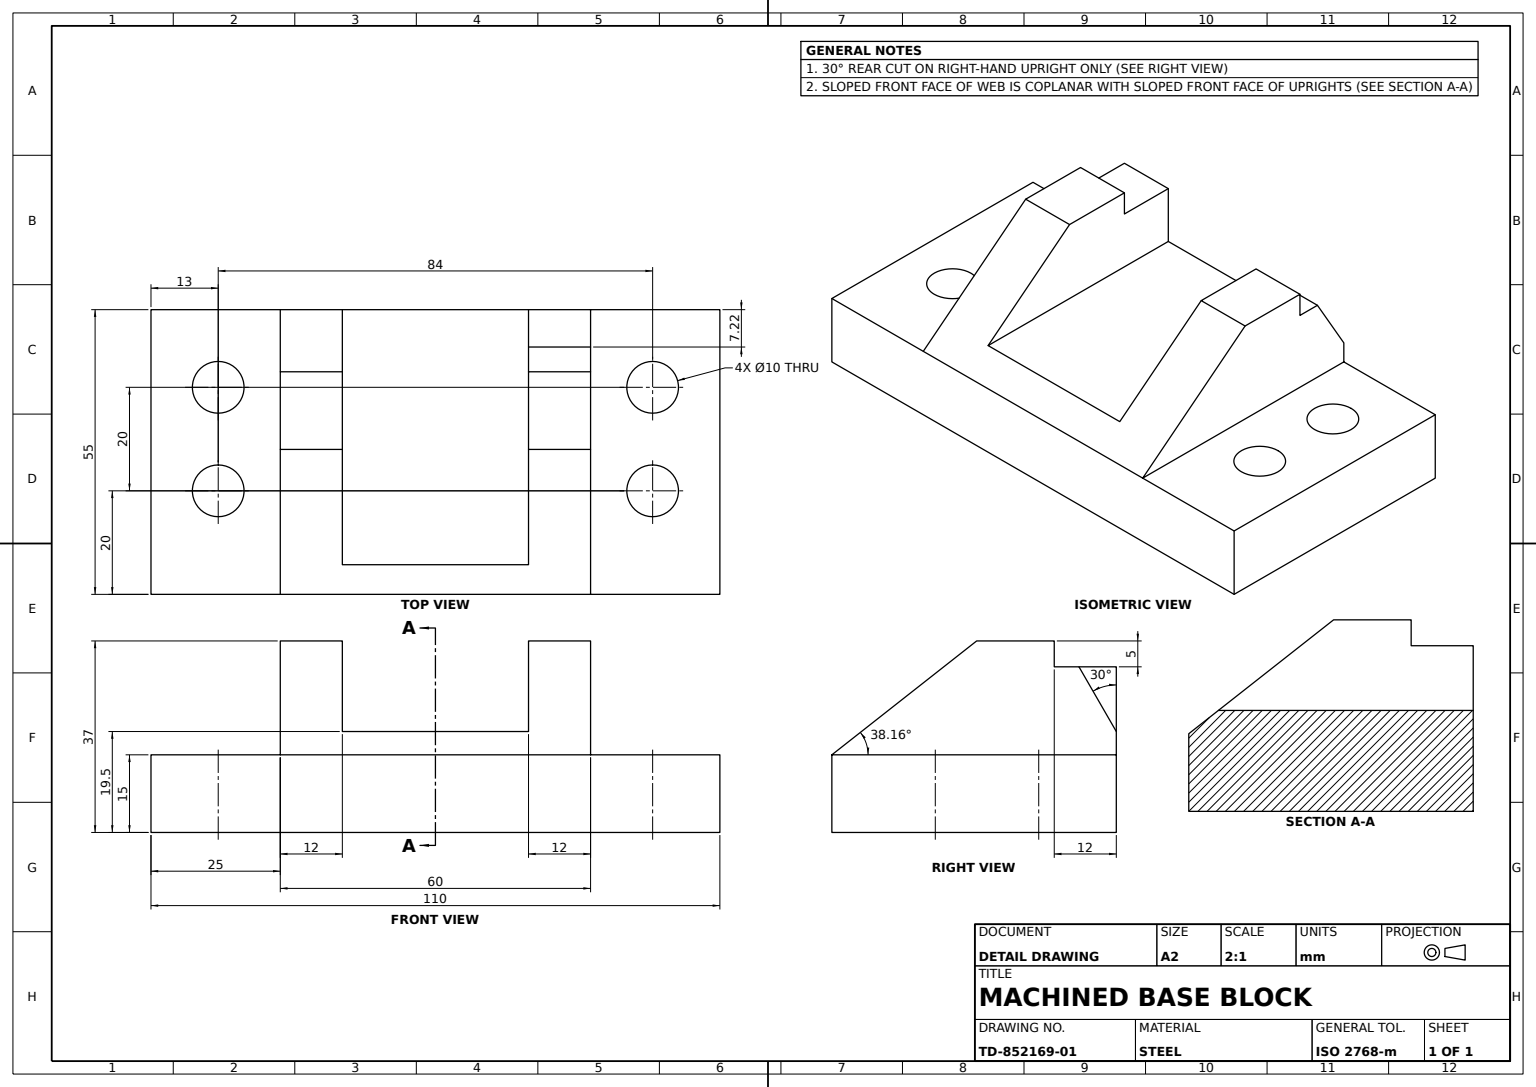
SolidWorks part; units mm, degrees
material "Plain Carbon Steel"
ref_plane "Front Plane" through (0, 0, 0) normal (0, 0, 1) x (1, 0, 0)
ref_plane "Top Plane" through (0, 0, 0) normal (0, 1, 0) x (1, 0, 0)
ref_plane "Right Plane" through (0, 0, 0) normal (1, 0, 0) x (0, 0, -1)
sketch "Base Plate Sketch" plane through (0, 0, 0) normal (0, 1, 0) x (1, 0, 0)
  line L0 (0, 55) -> (0, 0) construction
  line L1 (-55, 0) -> (55, 0)
  line L2 (-55, 0) -> (-55, 55)
  line L3 (-55, 55) -> (55, 55)
  line L4 (55, 0) -> (55, 55)
  line L5 (-42, 55) -> (-42, 0) construction
  circle A0 centre (-42, 40) radius 5
  circle A1 centre (-42, 20) radius 5
  circle A2 centre (42, 20) radius 5
  circle A3 centre (42, 40) radius 5
  point P4 (0, 0)
  dimension "D3" = 20
  dimension "D4" = 10
  dimension "D1" = 110
  dimension "D2" = 55
  dimension "D5" = 20
  dimension "D6" = 42
extrude "Base Plate" add sketch "Base Plate Sketch" along normal blind 15
sketch "V-Block Uprights Sketch" plane through (0, 0, -55) normal (0, 0, -1) x (-1, 0, 0)
  line L0 (0, 15) -> (0, 63.744) construction
  line L1 (-55, 15) -> (55, 15) construction
  line L2 (-30, 37) -> (30, 37) construction
  line L3 (-30, 15) -> (-18, 15)
  line L4 (-30, 15) -> (-30, 37)
  line L5 (-30, 37) -> (-18, 37)
  line L6 (-18, 19.5) -> (-18, 37)
  line L7 (18, 15) -> (30, 15)
  line L8 (18, 19.5) -> (18, 37)
  line L9 (18, 37) -> (30, 37)
  line L10 (30, 15) -> (30, 37)
  line L11 (18, 19.5) -> (-18, 19.5)
  line L12 (18, 15) -> (-18, 15)
  line L14 (-55, 0) -> (55, 0) construction
  circle A0 centre (0, 37) radius 17.5 construction
  point P18 (0, 19.5)
  point P20 (0, 15)
  dimension "D5" = 35
  dimension "D1" = 22
  dimension "D2" = 12
  dimension "D3" = 12
  dimension "D4" = 60
  dimension "D6" = 19.5
extrude "V-Block Uprights" add sketch "V-Block Uprights Sketch" against normal up to surface (55 mm away) up to face at (0, 7.5, 0)
sketch "Upright Notch Sketch" plane through (-30, 0, 0) normal (-1, 0, 0) x (0, 0, 1)
  line L0 (0, 15) -> (-28, 37)
  line L1 (0, 37) -> (-55, 37) construction
  line L2 (-28, 37) -> (0, 37)
  line L3 (0, 37) -> (0, 15)
  line L4 (-43, 37) -> (-43, 32)
  line L5 (-43, 32) -> (-55, 32)
  line L6 (-55, 15) -> (-55, 37) construction
  line L7 (-55, 32) -> (-55, 37)
  line L8 (-55, 37) -> (-43, 37)
  dimension "D1" = 5
  dimension "D2" = 12
  dimension "D3" = 27
extrude "Upright Notch" cut sketch "Upright Notch Sketch" against normal through all
sketch "Angled Cut 30deg Sketch" plane through (18, 0, 0) normal (-1, 0, 0) x (0, 0, 1)
  line L0 (-55, 19.5) -> (-47.7831, 32)
  line L1 (-55, 32) -> (-43, 32) construction
  line L2 (-47.7831, 32) -> (-55, 32)
  line L3 (-55, 32) -> (-55, 19.5)
  dimension "D1" = 30
extrude "Angled Cut 30deg" cut sketch "Angled Cut 30deg Sketch" against normal up to surface (12 mm away) contours L0 L2 L3 up to face at (30, 28, -37.3333)
